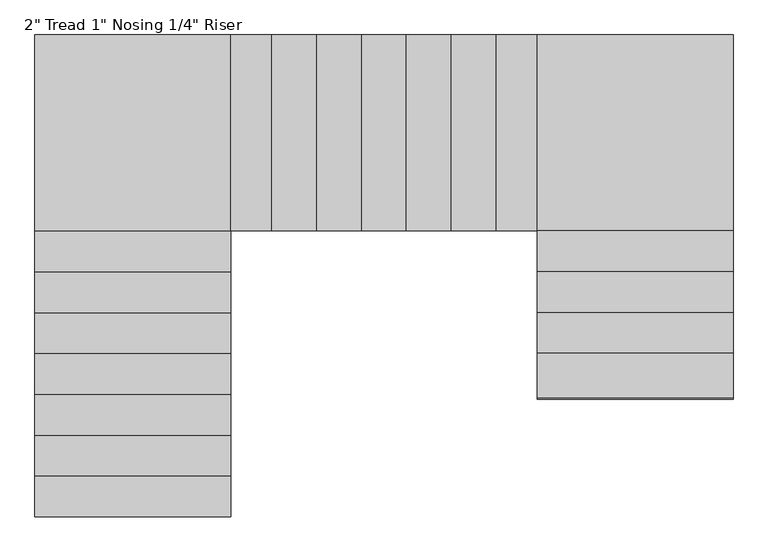
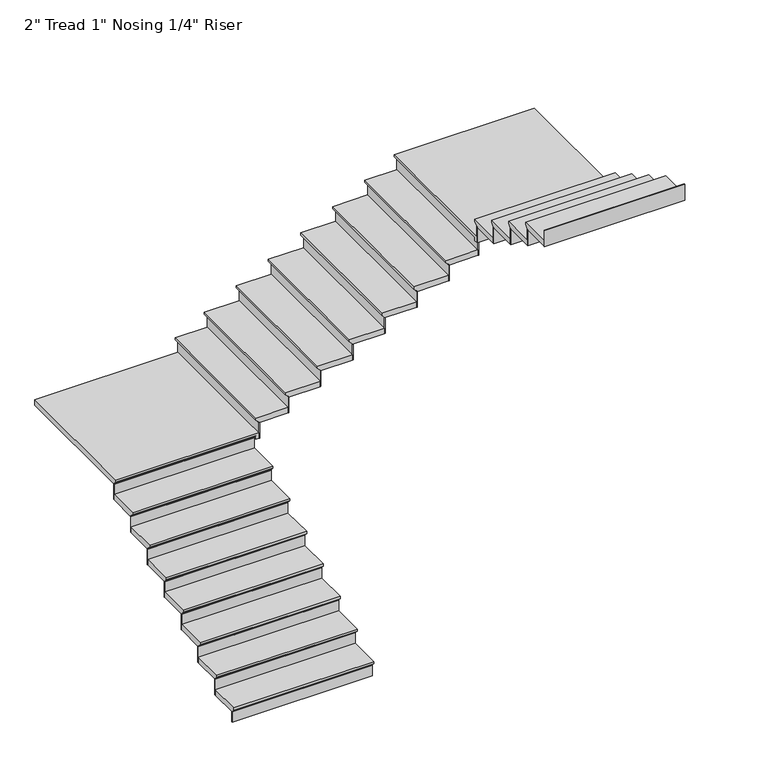
"""IFC4 building model written with IfcOpenShell, lengths in millimetres: stair flight geometry."""

from ifc_helpers import new_model, si_unit, origin, place, context, project, spatial, faceted_brep, source, transform, mapped, element, save


def stair_flight_6f949d0f(model_context):
    return source(origin(), model_context, "Body", "Brep", [
        faceted_brep([(-39782.5146233, 12459.3864709, 3174.0928571), (-39782.5146233, 12459.3864709, 3193.1428571), (-41001.7146233, 12459.3864709, 3193.1428571), (-41001.7146233, 12459.3864709, 3174.0928571), (-39782.5146233, 12484.7864709, 3148.6928571), (-41001.7146233, 12484.7864709, 3148.6928571), (-39782.5146233, 12738.7864709, 3193.1428571), (-41001.7146233, 12738.7864709, 3193.1428571), (-41001.7146233, 12484.7864709, 3142.3428571), (-41001.7146233, 12738.7864709, 3142.3428571), (-39782.5146233, 12738.7864709, 3142.3428571), (-39782.5146233, 12484.7864709, 3142.3428571)], [[[0, 1, 2, 3]], [[4, 0, 3, 5]], [[2, 1, 6, 7]], [[8, 9, 10, 11]], [[2, 7, 9, 8, 5, 3]], [[8, 11, 4, 5]], [[6, 1, 0, 4, 11, 10]], [[7, 6, 10, 9]]]),
        faceted_brep([(-39782.5146233, 12484.7864709, 3142.3428571), (-39782.5146233, 12484.7864709, 3048.0), (-39782.5146233, 12491.1364709, 3048.0), (-39782.5146233, 12491.1364709, 3142.3428571), (-41001.7146233, 12484.7864709, 3142.3428571), (-41001.7146233, 12491.1364709, 3142.3428571), (-41001.7146233, 12491.1364709, 3048.0), (-41001.7146233, 12484.7864709, 3048.0)], [[[0, 1, 2, 3]], [[4, 5, 6, 7]], [[1, 0, 4, 7]], [[2, 1, 7, 6]], [[3, 2, 6, 5]], [[0, 3, 5, 4]]]),
        faceted_brep([(-39782.5146233, 12738.7864709, 3287.4857143), (-39782.5146233, 12738.7864709, 3142.3428571), (-39782.5146233, 12745.1364709, 3142.3428571), (-39782.5146233, 12745.1364709, 3287.4857143), (-41001.7146233, 12738.7864709, 3287.4857143), (-41001.7146233, 12745.1364709, 3287.4857143), (-41001.7146233, 12745.1364709, 3142.3428571), (-41001.7146233, 12738.7864709, 3142.3428571)], [[[0, 1, 2, 3]], [[4, 5, 6, 7]], [[1, 0, 4, 7]], [[2, 1, 7, 6]], [[3, 2, 6, 5]], [[0, 3, 5, 4]]]),
        faceted_brep([(-41001.7146233, 12713.3864709, 3338.2857143), (-39782.5146233, 12713.3864709, 3338.2857143), (-39782.5146233, 12992.7864709, 3338.2857143), (-41001.7146233, 12992.7864709, 3338.2857143), (-41001.7146233, 12738.7864709, 3287.4857143), (-41001.7146233, 12992.7864709, 3287.4857143), (-39782.5146233, 12992.7864709, 3287.4857143), (-39782.5146233, 12738.7864709, 3287.4857143), (-41001.7146233, 12738.7864709, 3293.8357143), (-41001.7146233, 12713.3864709, 3319.2357143), (-39782.5146233, 12738.7864709, 3293.8357143), (-39782.5146233, 12713.3864709, 3319.2357143)], [[[0, 1, 2, 3]], [[4, 5, 6, 7]], [[0, 3, 5, 4, 8, 9]], [[4, 7, 10, 8]], [[2, 1, 11, 10, 7, 6]], [[3, 2, 6, 5]], [[11, 1, 0, 9]], [[10, 11, 9, 8]]]),
        faceted_brep([(-39782.5146233, 12992.7864709, 3432.6285714), (-39782.5146233, 12992.7864709, 3287.4857143), (-39782.5146233, 12999.1364709, 3287.4857143), (-39782.5146233, 12999.1364709, 3432.6285714), (-41001.7146233, 12992.7864709, 3432.6285714), (-41001.7146233, 12999.1364709, 3432.6285714), (-41001.7146233, 12999.1364709, 3287.4857143), (-41001.7146233, 12992.7864709, 3287.4857143)], [[[0, 1, 2, 3]], [[4, 5, 6, 7]], [[1, 0, 4, 7]], [[2, 1, 7, 6]], [[3, 2, 6, 5]], [[0, 3, 5, 4]]]),
        faceted_brep([(-41001.7146233, 12967.3864709, 3483.4285714), (-39782.5146233, 12967.3864709, 3483.4285714), (-39782.5146233, 13246.7864709, 3483.4285714), (-41001.7146233, 13246.7864709, 3483.4285714), (-41001.7146233, 12992.7864709, 3432.6285714), (-41001.7146233, 13246.7864709, 3432.6285714), (-39782.5146233, 13246.7864709, 3432.6285714), (-39782.5146233, 12992.7864709, 3432.6285714), (-41001.7146233, 12992.7864709, 3438.9785714), (-41001.7146233, 12967.3864709, 3464.3785714), (-39782.5146233, 12992.7864709, 3438.9785714), (-39782.5146233, 12967.3864709, 3464.3785714)], [[[0, 1, 2, 3]], [[4, 5, 6, 7]], [[0, 3, 5, 4, 8, 9]], [[4, 7, 10, 8]], [[2, 1, 11, 10, 7, 6]], [[3, 2, 6, 5]], [[11, 1, 0, 9]], [[10, 11, 9, 8]]]),
        faceted_brep([(-39782.5146233, 13246.7864709, 3577.7714286), (-39782.5146233, 13246.7864709, 3432.6285714), (-39782.5146233, 13253.1364709, 3432.6285714), (-39782.5146233, 13253.1364709, 3577.7714286), (-41001.7146233, 13246.7864709, 3577.7714286), (-41001.7146233, 13253.1364709, 3577.7714286), (-41001.7146233, 13253.1364709, 3432.6285714), (-41001.7146233, 13246.7864709, 3432.6285714)], [[[0, 1, 2, 3]], [[4, 5, 6, 7]], [[1, 0, 4, 7]], [[2, 1, 7, 6]], [[3, 2, 6, 5]], [[0, 3, 5, 4]]]),
        faceted_brep([(-41001.7146233, 13221.3864709, 3628.5714286), (-39782.5146233, 13221.3864709, 3628.5714286), (-39782.5146233, 13500.7864709, 3628.5714286), (-41001.7146233, 13500.7864709, 3628.5714286), (-41001.7146233, 13246.7864709, 3577.7714286), (-41001.7146233, 13500.7864709, 3577.7714286), (-39782.5146233, 13500.7864709, 3577.7714286), (-39782.5146233, 13246.7864709, 3577.7714286), (-41001.7146233, 13246.7864709, 3584.1214286), (-41001.7146233, 13221.3864709, 3609.5214286), (-39782.5146233, 13246.7864709, 3584.1214286), (-39782.5146233, 13221.3864709, 3609.5214286)], [[[0, 1, 2, 3]], [[4, 5, 6, 7]], [[0, 3, 5, 4, 8, 9]], [[4, 7, 10, 8]], [[2, 1, 11, 10, 7, 6]], [[3, 2, 6, 5]], [[11, 1, 0, 9]], [[10, 11, 9, 8]]]),
        faceted_brep([(-39782.5146233, 13500.7864709, 3722.9142857), (-39782.5146233, 13500.7864709, 3577.7714286), (-39782.5146233, 13507.1364709, 3577.7714286), (-39782.5146233, 13507.1364709, 3722.9142857), (-41001.7146233, 13500.7864709, 3722.9142857), (-41001.7146233, 13507.1364709, 3722.9142857), (-41001.7146233, 13507.1364709, 3577.7714286), (-41001.7146233, 13500.7864709, 3577.7714286)], [[[0, 1, 2, 3]], [[4, 5, 6, 7]], [[1, 0, 4, 7]], [[2, 1, 7, 6]], [[3, 2, 6, 5]], [[0, 3, 5, 4]]]),
        faceted_brep([(-41001.7146233, 13475.3864709, 3773.7142857), (-39782.5146233, 13475.3864709, 3773.7142857), (-39782.5146233, 13754.7864709, 3773.7142857), (-41001.7146233, 13754.7864709, 3773.7142857), (-41001.7146233, 13500.7864709, 3722.9142857), (-41001.7146233, 13754.7864709, 3722.9142857), (-39782.5146233, 13754.7864709, 3722.9142857), (-39782.5146233, 13500.7864709, 3722.9142857), (-41001.7146233, 13500.7864709, 3729.2642857), (-41001.7146233, 13475.3864709, 3754.6642857), (-39782.5146233, 13500.7864709, 3729.2642857), (-39782.5146233, 13475.3864709, 3754.6642857)], [[[0, 1, 2, 3]], [[4, 5, 6, 7]], [[0, 3, 5, 4, 8, 9]], [[4, 7, 10, 8]], [[2, 1, 11, 10, 7, 6]], [[3, 2, 6, 5]], [[11, 1, 0, 9]], [[10, 11, 9, 8]]]),
        faceted_brep([(-39782.5146233, 13754.7864709, 3868.0571429), (-39782.5146233, 13754.7864709, 3722.9142857), (-39782.5146233, 13761.1364709, 3722.9142857), (-39782.5146233, 13761.1364709, 3868.0571429), (-41001.7146233, 13754.7864709, 3868.0571429), (-41001.7146233, 13761.1364709, 3868.0571429), (-41001.7146233, 13761.1364709, 3722.9142857), (-41001.7146233, 13754.7864709, 3722.9142857)], [[[0, 1, 2, 3]], [[4, 5, 6, 7]], [[1, 0, 4, 7]], [[2, 1, 7, 6]], [[3, 2, 6, 5]], [[0, 3, 5, 4]]]),
        faceted_brep([(-41001.7146233, 13729.3864709, 3918.8571429), (-39782.5146233, 13729.3864709, 3918.8571429), (-39782.5146233, 14008.7864709, 3918.8571429), (-41001.7146233, 14008.7864709, 3918.8571429), (-41001.7146233, 13754.7864709, 3868.0571429), (-41001.7146233, 14008.7864709, 3868.0571429), (-39782.5146233, 14008.7864709, 3868.0571429), (-39782.5146233, 13754.7864709, 3868.0571429), (-41001.7146233, 13754.7864709, 3874.4071429), (-41001.7146233, 13729.3864709, 3899.8071429), (-39782.5146233, 13754.7864709, 3874.4071429), (-39782.5146233, 13729.3864709, 3899.8071429)], [[[0, 1, 2, 3]], [[4, 5, 6, 7]], [[0, 3, 5, 4, 8, 9]], [[4, 7, 10, 8]], [[2, 1, 11, 10, 7, 6]], [[3, 2, 6, 5]], [[11, 1, 0, 9]], [[10, 11, 9, 8]]]),
        faceted_brep([(-39782.5146233, 14008.7864709, 4013.2), (-39782.5146233, 14008.7864709, 3868.0571429), (-39782.5146233, 14015.1364709, 3868.0571429), (-39782.5146233, 14015.1364709, 4013.2), (-41001.7146233, 14008.7864709, 4013.2), (-41001.7146233, 14015.1364709, 4013.2), (-41001.7146233, 14015.1364709, 3868.0571429), (-41001.7146233, 14008.7864709, 3868.0571429)], [[[0, 1, 2, 3]], [[4, 5, 6, 7]], [[1, 0, 4, 7]], [[2, 1, 7, 6]], [[3, 2, 6, 5]], [[0, 3, 5, 4]]]),
        faceted_brep([(-41001.7146233, 13983.3864709, 4064.0), (-39782.5146233, 13983.3864709, 4064.0), (-39782.5146233, 14262.7864709, 4064.0), (-41001.7146233, 14262.7864709, 4064.0), (-41001.7146233, 14008.7864709, 4013.2), (-41001.7146233, 14262.7864709, 4013.2), (-39782.5146233, 14262.7864709, 4013.2), (-39782.5146233, 14008.7864709, 4013.2), (-41001.7146233, 14008.7864709, 4019.55), (-41001.7146233, 13983.3864709, 4044.95), (-39782.5146233, 14008.7864709, 4019.55), (-39782.5146233, 13983.3864709, 4044.95)], [[[0, 1, 2, 3]], [[4, 5, 6, 7]], [[0, 3, 5, 4, 8, 9]], [[4, 7, 10, 8]], [[2, 1, 11, 10, 7, 6]], [[3, 2, 6, 5]], [[11, 1, 0, 9]], [[10, 11, 9, 8]]]),
        faceted_brep([(-39782.5146233, 14262.7864709, 4158.3428571), (-39782.5146233, 14262.7864709, 4013.2), (-39782.5146233, 14269.1364709, 4013.2), (-39782.5146233, 14269.1364709, 4158.3428571), (-41001.7146233, 14262.7864709, 4158.3428571), (-41001.7146233, 14269.1364709, 4158.3428571), (-41001.7146233, 14269.1364709, 4013.2), (-41001.7146233, 14262.7864709, 4013.2)], [[[0, 1, 2, 3]], [[4, 5, 6, 7]], [[1, 0, 4, 7]], [[2, 1, 7, 6]], [[3, 2, 6, 5]], [[0, 3, 5, 4]]]),
        faceted_brep([(-39757.1146233, 15456.5864709, 4209.1428571), (-41001.7146233, 15456.5864709, 4209.1428571), (-41001.7146233, 14237.3864709, 4209.1428571), (-39757.1146233, 14237.3864709, 4209.1428571), (-41001.7146233, 15456.5864709, 4158.3428571), (-39757.1146233, 15456.5864709, 4158.3428571), (-39757.1146233, 14237.3864709, 4158.3428571), (-39782.5146233, 14237.3864709, 4158.3428571), (-39782.5146233, 14262.7864709, 4158.3428571), (-41001.7146233, 14262.7864709, 4158.3428571), (-41001.7146233, 14262.7864709, 4164.6928571), (-41001.7146233, 14237.3864709, 4190.0928571), (-39782.5146233, 14262.7864709, 4164.6928571), (-39782.5146233, 14237.3864709, 4190.0928571)], [[[0, 1, 2, 3]], [[4, 5, 6, 7, 8, 9]], [[1, 0, 5, 4]], [[2, 1, 4, 9, 10, 11]], [[9, 8, 12, 10]], [[8, 7, 13, 12]], [[3, 2, 11, 13, 7, 6]], [[0, 3, 6, 5]], [[11, 10, 12, 13]]]),
        faceted_brep([(-39757.1146233, 14237.3864709, 4303.4857143), (-39757.1146233, 14237.3864709, 4158.3428571), (-39750.7646233, 14237.3864709, 4158.3428571), (-39750.7646233, 14237.3864709, 4303.4857143), (-39757.1146233, 15456.5864709, 4303.4857143), (-39750.7646233, 15456.5864709, 4303.4857143), (-39750.7646233, 15456.5864709, 4158.3428571), (-39757.1146233, 15456.5864709, 4158.3428571)], [[[0, 1, 2, 3]], [[4, 5, 6, 7]], [[1, 0, 4, 7]], [[2, 1, 7, 6]], [[3, 2, 6, 5]], [[0, 3, 5, 4]]]),
        faceted_brep([(-39782.5146233, 15456.5864709, 4354.2857143), (-39782.5146233, 14237.3864709, 4354.2857143), (-39503.1146233, 14237.3864709, 4354.2857143), (-39503.1146233, 15456.5864709, 4354.2857143), (-39757.1146233, 15456.5864709, 4303.4857143), (-39503.1146233, 15456.5864709, 4303.4857143), (-39503.1146233, 14237.3864709, 4303.4857143), (-39757.1146233, 14237.3864709, 4303.4857143), (-39757.1146233, 15456.5864709, 4309.8357143), (-39782.5146233, 15456.5864709, 4335.2357143), (-39757.1146233, 14237.3864709, 4309.8357143), (-39782.5146233, 14237.3864709, 4335.2357143)], [[[0, 1, 2, 3]], [[4, 5, 6, 7]], [[0, 3, 5, 4, 8, 9]], [[4, 7, 10, 8]], [[2, 1, 11, 10, 7, 6]], [[3, 2, 6, 5]], [[11, 1, 0, 9]], [[10, 11, 9, 8]]]),
        faceted_brep([(-39503.1146233, 14237.3864709, 4448.6285714), (-39503.1146233, 14237.3864709, 4303.4857143), (-39496.7646233, 14237.3864709, 4303.4857143), (-39496.7646233, 14237.3864709, 4448.6285714), (-39503.1146233, 15456.5864709, 4448.6285714), (-39496.7646233, 15456.5864709, 4448.6285714), (-39496.7646233, 15456.5864709, 4303.4857143), (-39503.1146233, 15456.5864709, 4303.4857143)], [[[0, 1, 2, 3]], [[4, 5, 6, 7]], [[1, 0, 4, 7]], [[2, 1, 7, 6]], [[3, 2, 6, 5]], [[0, 3, 5, 4]]]),
        faceted_brep([(-39528.5146233, 15456.5864709, 4499.4285714), (-39528.5146233, 14237.3864709, 4499.4285714), (-39223.7146233, 14237.3864709, 4499.4285714), (-39223.7146233, 15456.5864709, 4499.4285714), (-39503.1146233, 15456.5864709, 4448.6285714), (-39223.7146233, 15456.5864709, 4448.6285714), (-39223.7146233, 14237.3864709, 4448.6285714), (-39503.1146233, 14237.3864709, 4448.6285714), (-39503.1146233, 15456.5864709, 4454.9785714), (-39528.5146233, 15456.5864709, 4480.3785714), (-39503.1146233, 14237.3864709, 4454.9785714), (-39528.5146233, 14237.3864709, 4480.3785714)], [[[0, 1, 2, 3]], [[4, 5, 6, 7]], [[0, 3, 5, 4, 8, 9]], [[4, 7, 10, 8]], [[2, 1, 11, 10, 7, 6]], [[3, 2, 6, 5]], [[11, 1, 0, 9]], [[10, 11, 9, 8]]]),
        faceted_brep([(-39223.7146233, 14237.3864709, 4593.7714286), (-39223.7146233, 14237.3864709, 4448.6285714), (-39217.3646233, 14237.3864709, 4448.6285714), (-39217.3646233, 14237.3864709, 4593.7714286), (-39223.7146233, 15456.5864709, 4593.7714286), (-39217.3646233, 15456.5864709, 4593.7714286), (-39217.3646233, 15456.5864709, 4448.6285714), (-39223.7146233, 15456.5864709, 4448.6285714)], [[[0, 1, 2, 3]], [[4, 5, 6, 7]], [[1, 0, 4, 7]], [[2, 1, 7, 6]], [[3, 2, 6, 5]], [[0, 3, 5, 4]]]),
        faceted_brep([(-39249.1146233, 15456.5864709, 4644.5714286), (-39249.1146233, 14237.3864709, 4644.5714286), (-38944.3146233, 14237.3864709, 4644.5714286), (-38944.3146233, 15456.5864709, 4644.5714286), (-39223.7146233, 15456.5864709, 4593.7714286), (-38944.3146233, 15456.5864709, 4593.7714286), (-38944.3146233, 14237.3864709, 4593.7714286), (-39223.7146233, 14237.3864709, 4593.7714286), (-39223.7146233, 15456.5864709, 4600.1214286), (-39249.1146233, 15456.5864709, 4625.5214286), (-39223.7146233, 14237.3864709, 4600.1214286), (-39249.1146233, 14237.3864709, 4625.5214286)], [[[0, 1, 2, 3]], [[4, 5, 6, 7]], [[0, 3, 5, 4, 8, 9]], [[4, 7, 10, 8]], [[2, 1, 11, 10, 7, 6]], [[3, 2, 6, 5]], [[11, 1, 0, 9]], [[10, 11, 9, 8]]]),
        faceted_brep([(-38944.3146233, 14237.3864709, 4738.9142857), (-38944.3146233, 14237.3864709, 4593.7714286), (-38937.9646233, 14237.3864709, 4593.7714286), (-38937.9646233, 14237.3864709, 4738.9142857), (-38944.3146233, 15456.5864709, 4738.9142857), (-38937.9646233, 15456.5864709, 4738.9142857), (-38937.9646233, 15456.5864709, 4593.7714286), (-38944.3146233, 15456.5864709, 4593.7714286)], [[[0, 1, 2, 3]], [[4, 5, 6, 7]], [[1, 0, 4, 7]], [[2, 1, 7, 6]], [[3, 2, 6, 5]], [[0, 3, 5, 4]]]),
        faceted_brep([(-38969.7146233, 15456.5864709, 4789.7142857), (-38969.7146233, 14237.3864709, 4789.7142857), (-38664.9146233, 14237.3864709, 4789.7142857), (-38664.9146233, 15456.5864709, 4789.7142857), (-38944.3146233, 15456.5864709, 4738.9142857), (-38664.9146233, 15456.5864709, 4738.9142857), (-38664.9146233, 14237.3864709, 4738.9142857), (-38944.3146233, 14237.3864709, 4738.9142857), (-38944.3146233, 15456.5864709, 4745.2642857), (-38969.7146233, 15456.5864709, 4770.6642857), (-38944.3146233, 14237.3864709, 4745.2642857), (-38969.7146233, 14237.3864709, 4770.6642857)], [[[0, 1, 2, 3]], [[4, 5, 6, 7]], [[0, 3, 5, 4, 8, 9]], [[4, 7, 10, 8]], [[2, 1, 11, 10, 7, 6]], [[3, 2, 6, 5]], [[11, 1, 0, 9]], [[10, 11, 9, 8]]]),
        faceted_brep([(-38664.9146233, 14237.3864709, 4884.0571429), (-38664.9146233, 14237.3864709, 4738.9142857), (-38658.5646233, 14237.3864709, 4738.9142857), (-38658.5646233, 14237.3864709, 4884.0571429), (-38664.9146233, 15456.5864709, 4884.0571429), (-38658.5646233, 15456.5864709, 4884.0571429), (-38658.5646233, 15456.5864709, 4738.9142857), (-38664.9146233, 15456.5864709, 4738.9142857)], [[[0, 1, 2, 3]], [[4, 5, 6, 7]], [[1, 0, 4, 7]], [[2, 1, 7, 6]], [[3, 2, 6, 5]], [[0, 3, 5, 4]]]),
        faceted_brep([(-38690.3146233, 15456.5864709, 4934.8571429), (-38690.3146233, 14237.3864709, 4934.8571429), (-38385.5146233, 14237.3864709, 4934.8571429), (-38385.5146233, 15456.5864709, 4934.8571429), (-38664.9146233, 15456.5864709, 4884.0571429), (-38385.5146233, 15456.5864709, 4884.0571429), (-38385.5146233, 14237.3864709, 4884.0571429), (-38664.9146233, 14237.3864709, 4884.0571429), (-38664.9146233, 15456.5864709, 4890.4071429), (-38690.3146233, 15456.5864709, 4915.8071429), (-38664.9146233, 14237.3864709, 4890.4071429), (-38690.3146233, 14237.3864709, 4915.8071429)], [[[0, 1, 2, 3]], [[4, 5, 6, 7]], [[0, 3, 5, 4, 8, 9]], [[4, 7, 10, 8]], [[2, 1, 11, 10, 7, 6]], [[3, 2, 6, 5]], [[11, 1, 0, 9]], [[10, 11, 9, 8]]]),
        faceted_brep([(-38385.5146233, 14237.3864709, 5029.2), (-38385.5146233, 14237.3864709, 4884.0571429), (-38379.1646233, 14237.3864709, 4884.0571429), (-38379.1646233, 14237.3864709, 5029.2), (-38385.5146233, 15456.5864709, 5029.2), (-38379.1646233, 15456.5864709, 5029.2), (-38379.1646233, 15456.5864709, 4884.0571429), (-38385.5146233, 15456.5864709, 4884.0571429)], [[[0, 1, 2, 3]], [[4, 5, 6, 7]], [[1, 0, 4, 7]], [[2, 1, 7, 6]], [[3, 2, 6, 5]], [[0, 3, 5, 4]]]),
        faceted_brep([(-38410.9146233, 15456.5864709, 5080.0), (-38410.9146233, 14237.3864709, 5080.0), (-38106.1146233, 14237.3864709, 5080.0), (-38106.1146233, 15456.5864709, 5080.0), (-38385.5146233, 15456.5864709, 5029.2), (-38106.1146233, 15456.5864709, 5029.2), (-38106.1146233, 14237.3864709, 5029.2), (-38385.5146233, 14237.3864709, 5029.2), (-38385.5146233, 15456.5864709, 5035.55), (-38410.9146233, 15456.5864709, 5060.95), (-38385.5146233, 14237.3864709, 5035.55), (-38410.9146233, 14237.3864709, 5060.95)], [[[0, 1, 2, 3]], [[4, 5, 6, 7]], [[0, 3, 5, 4, 8, 9]], [[4, 7, 10, 8]], [[2, 1, 11, 10, 7, 6]], [[3, 2, 6, 5]], [[11, 1, 0, 9]], [[10, 11, 9, 8]]]),
        faceted_brep([(-38106.1146233, 14237.3864709, 5174.3428571), (-38106.1146233, 14237.3864709, 5029.2), (-38099.7646233, 14237.3864709, 5029.2), (-38099.7646233, 14237.3864709, 5174.3428571), (-38106.1146233, 15456.5864709, 5174.3428571), (-38099.7646233, 15456.5864709, 5174.3428571), (-38099.7646233, 15456.5864709, 5029.2), (-38106.1146233, 15456.5864709, 5029.2)], [[[0, 1, 2, 3]], [[4, 5, 6, 7]], [[1, 0, 4, 7]], [[2, 1, 7, 6]], [[3, 2, 6, 5]], [[0, 3, 5, 4]]]),
        faceted_brep([(-38131.5146233, 15456.5864709, 5225.1428571), (-38131.5146233, 14237.3864709, 5225.1428571), (-37852.1146233, 14237.3864709, 5225.1428571), (-37852.1146233, 15456.5864709, 5225.1428571), (-38106.1146233, 15456.5864709, 5174.3428571), (-37852.1146233, 15456.5864709, 5174.3428571), (-37852.1146233, 14237.3864709, 5174.3428571), (-38106.1146233, 14237.3864709, 5174.3428571), (-38106.1146233, 15456.5864709, 5180.6928571), (-38131.5146233, 15456.5864709, 5206.0928571), (-38106.1146233, 14237.3864709, 5180.6928571), (-38131.5146233, 14237.3864709, 5206.0928571)], [[[0, 1, 2, 3]], [[4, 5, 6, 7]], [[0, 3, 5, 4, 8, 9]], [[4, 7, 10, 8]], [[2, 1, 11, 10, 7, 6]], [[3, 2, 6, 5]], [[11, 1, 0, 9]], [[10, 11, 9, 8]]]),
        faceted_brep([(-37852.1146233, 14237.3864709, 5319.4857143), (-37852.1146233, 14237.3864709, 5174.3428571), (-37845.7646233, 14237.3864709, 5174.3428571), (-37845.7646233, 14237.3864709, 5319.4857143), (-37852.1146233, 15456.5864709, 5319.4857143), (-37845.7646233, 15456.5864709, 5319.4857143), (-37845.7646233, 15456.5864709, 5174.3428571), (-37852.1146233, 15456.5864709, 5174.3428571)], [[[0, 1, 2, 3]], [[4, 5, 6, 7]], [[1, 0, 4, 7]], [[2, 1, 7, 6]], [[3, 2, 6, 5]], [[0, 3, 5, 4]]]),
        faceted_brep([(-36658.3146233, 14211.9864709, 5370.2857143), (-36658.3146233, 15456.5864709, 5370.2857143), (-37877.5146233, 15456.5864709, 5370.2857143), (-37877.5146233, 14211.9864709, 5370.2857143), (-36658.3146233, 15456.5864709, 5319.4857143), (-36658.3146233, 14211.9864709, 5319.4857143), (-37877.5146233, 14211.9864709, 5319.4857143), (-37877.5146233, 14237.3864709, 5319.4857143), (-37852.1146233, 14237.3864709, 5319.4857143), (-37852.1146233, 15456.5864709, 5319.4857143), (-37852.1146233, 15456.5864709, 5325.8357143), (-37877.5146233, 15456.5864709, 5351.2357143), (-37852.1146233, 14237.3864709, 5325.8357143), (-37877.5146233, 14237.3864709, 5351.2357143)], [[[0, 1, 2, 3]], [[4, 5, 6, 7, 8, 9]], [[1, 0, 5, 4]], [[2, 1, 4, 9, 10, 11]], [[9, 8, 12, 10]], [[8, 7, 13, 12]], [[3, 2, 11, 13, 7, 6]], [[0, 3, 6, 5]], [[11, 10, 12, 13]]]),
        faceted_brep([(-37877.5146233, 14211.9864709, 5464.6285714), (-37877.5146233, 14211.9864709, 5319.4857143), (-37877.5146233, 14205.6364709, 5319.4857143), (-37877.5146233, 14205.6364709, 5464.6285714), (-36658.3146233, 14211.9864709, 5464.6285714), (-36658.3146233, 14205.6364709, 5464.6285714), (-36658.3146233, 14205.6364709, 5319.4857143), (-36658.3146233, 14211.9864709, 5319.4857143)], [[[0, 1, 2, 3]], [[4, 5, 6, 7]], [[1, 0, 4, 7]], [[2, 1, 7, 6]], [[3, 2, 6, 5]], [[0, 3, 5, 4]]]),
        faceted_brep([(-36658.3146233, 14237.3864709, 5515.4285714), (-37877.5146233, 14237.3864709, 5515.4285714), (-37877.5146233, 13957.9864709, 5515.4285714), (-36658.3146233, 13957.9864709, 5515.4285714), (-36658.3146233, 14211.9864709, 5464.6285714), (-36658.3146233, 13957.9864709, 5464.6285714), (-37877.5146233, 13957.9864709, 5464.6285714), (-37877.5146233, 14211.9864709, 5464.6285714), (-36658.3146233, 14211.9864709, 5470.9785714), (-36658.3146233, 14237.3864709, 5496.3785714), (-37877.5146233, 14211.9864709, 5470.9785714), (-37877.5146233, 14237.3864709, 5496.3785714)], [[[0, 1, 2, 3]], [[4, 5, 6, 7]], [[0, 3, 5, 4, 8, 9]], [[4, 7, 10, 8]], [[2, 1, 11, 10, 7, 6]], [[3, 2, 6, 5]], [[11, 1, 0, 9]], [[10, 11, 9, 8]]]),
        faceted_brep([(-37877.5146233, 13957.9864709, 5609.7714286), (-37877.5146233, 13957.9864709, 5464.6285714), (-37877.5146233, 13951.6364709, 5464.6285714), (-37877.5146233, 13951.6364709, 5609.7714286), (-36658.3146233, 13957.9864709, 5609.7714286), (-36658.3146233, 13951.6364709, 5609.7714286), (-36658.3146233, 13951.6364709, 5464.6285714), (-36658.3146233, 13957.9864709, 5464.6285714)], [[[0, 1, 2, 3]], [[4, 5, 6, 7]], [[1, 0, 4, 7]], [[2, 1, 7, 6]], [[3, 2, 6, 5]], [[0, 3, 5, 4]]]),
        faceted_brep([(-36658.3146233, 13983.3864709, 5660.5714286), (-37877.5146233, 13983.3864709, 5660.5714286), (-37877.5146233, 13703.9864709, 5660.5714286), (-36658.3146233, 13703.9864709, 5660.5714286), (-36658.3146233, 13957.9864709, 5609.7714286), (-36658.3146233, 13703.9864709, 5609.7714286), (-37877.5146233, 13703.9864709, 5609.7714286), (-37877.5146233, 13957.9864709, 5609.7714286), (-36658.3146233, 13957.9864709, 5616.1214286), (-36658.3146233, 13983.3864709, 5641.5214286), (-37877.5146233, 13957.9864709, 5616.1214286), (-37877.5146233, 13983.3864709, 5641.5214286)], [[[0, 1, 2, 3]], [[4, 5, 6, 7]], [[0, 3, 5, 4, 8, 9]], [[4, 7, 10, 8]], [[2, 1, 11, 10, 7, 6]], [[3, 2, 6, 5]], [[11, 1, 0, 9]], [[10, 11, 9, 8]]]),
        faceted_brep([(-37877.5146233, 13703.9864709, 5754.9142857), (-37877.5146233, 13703.9864709, 5609.7714286), (-37877.5146233, 13697.6364709, 5609.7714286), (-37877.5146233, 13697.6364709, 5754.9142857), (-36658.3146233, 13703.9864709, 5754.9142857), (-36658.3146233, 13697.6364709, 5754.9142857), (-36658.3146233, 13697.6364709, 5609.7714286), (-36658.3146233, 13703.9864709, 5609.7714286)], [[[0, 1, 2, 3]], [[4, 5, 6, 7]], [[1, 0, 4, 7]], [[2, 1, 7, 6]], [[3, 2, 6, 5]], [[0, 3, 5, 4]]]),
        faceted_brep([(-36658.3146233, 13729.3864709, 5805.7142857), (-37877.5146233, 13729.3864709, 5805.7142857), (-37877.5146233, 13449.9864709, 5805.7142857), (-36658.3146233, 13449.9864709, 5805.7142857), (-36658.3146233, 13703.9864709, 5754.9142857), (-36658.3146233, 13449.9864709, 5754.9142857), (-37877.5146233, 13449.9864709, 5754.9142857), (-37877.5146233, 13703.9864709, 5754.9142857), (-36658.3146233, 13703.9864709, 5761.2642857), (-36658.3146233, 13729.3864709, 5786.6642857), (-37877.5146233, 13703.9864709, 5761.2642857), (-37877.5146233, 13729.3864709, 5786.6642857)], [[[0, 1, 2, 3]], [[4, 5, 6, 7]], [[0, 3, 5, 4, 8, 9]], [[4, 7, 10, 8]], [[2, 1, 11, 10, 7, 6]], [[3, 2, 6, 5]], [[11, 1, 0, 9]], [[10, 11, 9, 8]]]),
        faceted_brep([(-37877.5146233, 13449.9864709, 5900.0571429), (-37877.5146233, 13449.9864709, 5754.9142857), (-37877.5146233, 13443.6364709, 5754.9142857), (-37877.5146233, 13443.6364709, 5900.0571429), (-36658.3146233, 13449.9864709, 5900.0571429), (-36658.3146233, 13443.6364709, 5900.0571429), (-36658.3146233, 13443.6364709, 5754.9142857), (-36658.3146233, 13449.9864709, 5754.9142857)], [[[0, 1, 2, 3]], [[4, 5, 6, 7]], [[1, 0, 4, 7]], [[2, 1, 7, 6]], [[3, 2, 6, 5]], [[0, 3, 5, 4]]]),
        faceted_brep([(-37877.5146233, 13195.9864709, 6045.2), (-37877.5146233, 13195.9864709, 5900.0571429), (-37877.5146233, 13189.6364709, 5900.0571429), (-37877.5146233, 13189.6364709, 6045.2), (-36658.3146233, 13195.9864709, 6045.2), (-36658.3146233, 13189.6364709, 6045.2), (-36658.3146233, 13189.6364709, 5900.0571429), (-36658.3146233, 13195.9864709, 5900.0571429)], [[[0, 1, 2, 3]], [[4, 5, 6, 7]], [[1, 0, 4, 7]], [[2, 1, 7, 6]], [[3, 2, 6, 5]], [[0, 3, 5, 4]]]),
        faceted_brep([(-36658.3146233, 13475.3864709, 5950.8571429), (-37877.5146233, 13475.3864709, 5950.8571429), (-37877.5146233, 13195.9864709, 5950.8571429), (-36658.3146233, 13195.9864709, 5950.8571429), (-36658.3146233, 13449.9864709, 5900.0571429), (-36658.3146233, 13195.9864709, 5900.0571429), (-37877.5146233, 13195.9864709, 5900.0571429), (-37877.5146233, 13449.9864709, 5900.0571429), (-36658.3146233, 13449.9864709, 5906.4071429), (-36658.3146233, 13475.3864709, 5931.8071429), (-37877.5146233, 13449.9864709, 5906.4071429), (-37877.5146233, 13475.3864709, 5931.8071429)], [[[0, 1, 2, 3]], [[4, 5, 6, 7]], [[0, 3, 5, 4, 8, 9]], [[4, 7, 10, 8]], [[2, 1, 11, 10, 7, 6]], [[3, 2, 6, 5]], [[11, 1, 0, 9]], [[10, 11, 9, 8]]]),
    ])


if __name__ == "__main__":
    model = new_model("IFC4")
    model_context = context("Model", 3, world=origin())
    ifc_project = project(units=[si_unit("LENGTHUNIT", "METRE", prefix="MILLI")], contexts=[model_context])
    site = spatial("IfcSite", under=ifc_project)
    building = spatial("IfcBuilding", under=site)
    placement = place(None, origin())
    stair_flight_shape = stair_flight_6f949d0f(model_context)
    element("IfcStairFlight", 1, ObjectType="2\" Tread 1\" Nosing 1/4\" Riser", at=placement, inside=building, context=model_context, shape_type="MappedRepresentation", body=[
        mapped(stair_flight_shape, transform((0.0, 0.0, 0.0), x_axis=(1.0, 0.0, 0.0), y_axis=(0.0, 1.0, 0.0), z_axis=(0.0, 0.0, 1.0))),
    ])
    save(model, "model.ifc")
